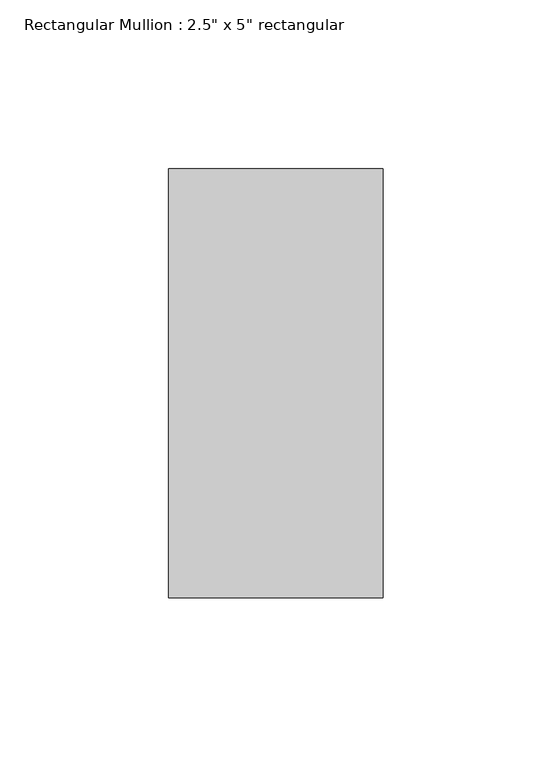
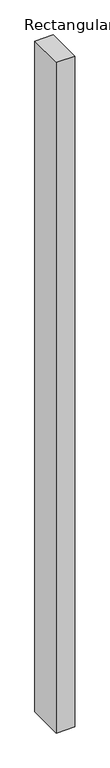
"""IFC4 building model written with IfcOpenShell, lengths in millimetres: member geometry."""

from ifc_helpers import new_model, si_unit, frame, origin, place, context, project, spatial, polyline, outline, extrude, source, transform, mapped, element, save


def member_f0fea5a5(model_context):
    return source(origin(), model_context, "Body", "SweptSolid", [
        extrude(outline(polyline([(31.75, 63.5), (31.75, -63.5), (-31.75, -63.5), (-31.75, 63.5), (31.75, 63.5)])), frame((0.0, 0.0, -2438.4), z_axis=(0.0, 0.0, 1.0), x_axis=(1.0, 0.0, 0.0)), (0.0, 0.0, 1.0), 2438.4),
    ])


if __name__ == "__main__":
    model = new_model("IFC4")
    model_context = context("Model", 3, world=origin())
    ifc_project = project(units=[si_unit("LENGTHUNIT", "METRE", prefix="MILLI")], contexts=[model_context])
    site = spatial("IfcSite", under=ifc_project)
    building = spatial("IfcBuilding", under=site)
    placement = place(None, origin())
    member_shape = member_f0fea5a5(model_context)
    element("IfcMember", 1, ObjectType="Rectangular Mullion : 2.5\" x 5\" rectangular", at=placement, inside=building, context=model_context, shape_type="MappedRepresentation", body=[
        mapped(member_shape, transform((0.0, 0.0, 0.0), x_axis=(1.0, 0.0, 0.0), y_axis=(0.0, 1.0, 0.0), z_axis=(0.0, 0.0, 1.0))),
    ])
    save(model, "model.ifc")

# Revit data of these elements
# Type "Rectangular Mullion : 2.5\" x 5\" rectangular"
#   built-in parameter 1007304 = 0.416667 (stored number, unit not read)
#   built-in parameter 1007301 = 0.104167 (stored number, unit not read)
#   built-in parameter 1007300 = 0.104167 (stored number, unit not read)
# Element 1 (IfcMember, "Rectangular Mullion : 2.5\" x 5\" rectangular")
#   Materials on its faces: "WINDOW FRAMING"
# Materials
#   "WINDOW FRAMING": class "Generic", colour RGB 120 120 120, transparency 0, Cost = 0
